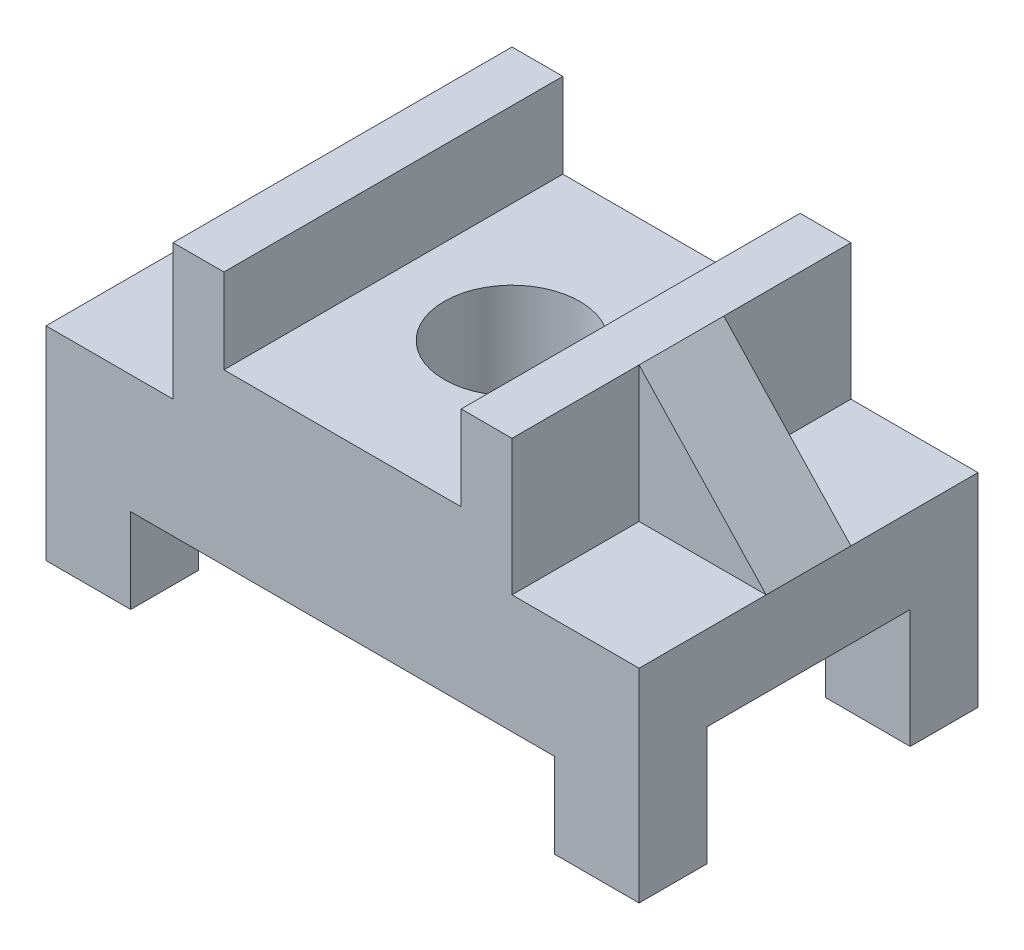
ISO-10303-21;
HEADER;
FILE_DESCRIPTION(('STEP AP214'),'2;1');
FILE_NAME('part.step','',(''),(''),'','','');
FILE_SCHEMA(('AUTOMOTIVE_DESIGN { 1 0 10303 214 1 1 1 1 }'));
ENDSEC;
DATA;
#1=APPLICATION_CONTEXT('core data for automotive mechanical design processes');
#2=APPLICATION_PROTOCOL_DEFINITION('international standard','automotive_design',2000,#1);
#3=PRODUCT_CONTEXT('',#1,'mechanical');
#4=PRODUCT('Part','Part','',(#3));
#5=PRODUCT_RELATED_PRODUCT_CATEGORY('part','',(#4));
#6=PRODUCT_DEFINITION_FORMATION('','',#4);
#7=PRODUCT_DEFINITION_CONTEXT('part definition',#1,'design');
#8=PRODUCT_DEFINITION('design','',#6,#7);
#9=PRODUCT_DEFINITION_SHAPE('','',#8);
#10=(LENGTH_UNIT() NAMED_UNIT(*) SI_UNIT(.MILLI.,.METRE.));
#11=(NAMED_UNIT(*) PLANE_ANGLE_UNIT() SI_UNIT($,.RADIAN.));
#12=(NAMED_UNIT(*) SI_UNIT($,.STERADIAN.) SOLID_ANGLE_UNIT());
#13=UNCERTAINTY_MEASURE_WITH_UNIT(LENGTH_MEASURE(1.E-05),#10,'distance_accuracy_value','');
#14=(GEOMETRIC_REPRESENTATION_CONTEXT(3) GLOBAL_UNCERTAINTY_ASSIGNED_CONTEXT((#13)) GLOBAL_UNIT_ASSIGNED_CONTEXT((#10,
#11,#12)) REPRESENTATION_CONTEXT('',''));
#15=CARTESIAN_POINT('',(0.,0.,0.));
#16=DIRECTION('',(0.,0.,1.));
#17=DIRECTION('',(1.,0.,0.));
#18=AXIS2_PLACEMENT_3D('',#15,#16,#17);
#19=CARTESIAN_POINT('',(0.,40.,20.));
#20=DIRECTION('',(0.,0.,-1.));
#21=DIRECTION('',(-1.,0.,0.));
#22=AXIS2_PLACEMENT_3D('',#19,#20,#21);
#23=PLANE('',#22);
#24=DIRECTION('',(0.,-1.,0.));
#25=VECTOR('',#24,1.);
#26=CARTESIAN_POINT('',(-25.,40.,20.));
#27=LINE('',#26,#25);
#28=CARTESIAN_POINT('',(-25.,10.,20.));
#29=VERTEX_POINT('',#28);
#30=CARTESIAN_POINT('',(-25.,0.,20.));
#31=VERTEX_POINT('',#30);
#32=EDGE_CURVE('E256',#29,#31,#27,.T.);
#33=ORIENTED_EDGE('',*,*,#32,.F.);
#34=DIRECTION('',(-1.,0.,0.));
#35=VECTOR('',#34,1.);
#36=CARTESIAN_POINT('',(0.,9.99999999999999,20.));
#37=LINE('',#36,#35);
#38=CARTESIAN_POINT('',(25.,10.,20.));
#39=VERTEX_POINT('',#38);
#40=EDGE_CURVE('E242',#39,#29,#37,.T.);
#41=ORIENTED_EDGE('',*,*,#40,.F.);
#42=DIRECTION('',(0.,1.,0.));
#43=VECTOR('',#42,1.);
#44=CARTESIAN_POINT('',(25.,40.,20.));
#45=LINE('',#44,#43);
#46=CARTESIAN_POINT('',(25.,0.,20.));
#47=VERTEX_POINT('',#46);
#48=EDGE_CURVE('E240',#47,#39,#45,.T.);
#49=ORIENTED_EDGE('',*,*,#48,.F.);
#50=DIRECTION('',(1.,0.,0.));
#51=VECTOR('',#50,1.);
#52=CARTESIAN_POINT('',(0.,0.,20.));
#53=LINE('',#52,#51);
#54=CARTESIAN_POINT('',(35.,0.,20.));
#55=VERTEX_POINT('',#54);
#56=EDGE_CURVE('E418',#47,#55,#53,.T.);
#57=ORIENTED_EDGE('',*,*,#56,.T.);
#58=DIRECTION('',(0.,-1.,0.));
#59=VECTOR('',#58,1.);
#60=CARTESIAN_POINT('',(35.,40.,20.));
#61=LINE('',#60,#59);
#62=CARTESIAN_POINT('',(35.,24.,20.));
#63=VERTEX_POINT('',#62);
#64=EDGE_CURVE('E432',#63,#55,#61,.T.);
#65=ORIENTED_EDGE('',*,*,#64,.F.);
#66=DIRECTION('',(1.,0.,0.));
#67=VECTOR('',#66,1.);
#68=CARTESIAN_POINT('',(0.,24.,20.));
#69=LINE('',#68,#67);
#70=CARTESIAN_POINT('',(20.,24.,20.));
#71=VERTEX_POINT('',#70);
#72=EDGE_CURVE('E360',#71,#63,#69,.T.);
#73=ORIENTED_EDGE('',*,*,#72,.F.);
#74=DIRECTION('',(0.,-1.,0.));
#75=VECTOR('',#74,1.);
#76=CARTESIAN_POINT('',(20.,40.,20.));
#77=LINE('',#76,#75);
#78=CARTESIAN_POINT('',(20.,40.,20.));
#79=VERTEX_POINT('',#78);
#80=EDGE_CURVE('E353',#79,#71,#77,.T.);
#81=ORIENTED_EDGE('',*,*,#80,.F.);
#82=DIRECTION('',(1.,0.,0.));
#83=VECTOR('',#82,1.);
#84=CARTESIAN_POINT('',(0.,40.,20.));
#85=LINE('',#84,#83);
#86=CARTESIAN_POINT('',(14.,40.,20.));
#87=VERTEX_POINT('',#86);
#88=EDGE_CURVE('E415',#87,#79,#85,.T.);
#89=ORIENTED_EDGE('',*,*,#88,.F.);
#90=DIRECTION('',(0.,1.,0.));
#91=VECTOR('',#90,1.);
#92=CARTESIAN_POINT('',(14.,0.,20.));
#93=LINE('',#92,#91);
#94=CARTESIAN_POINT('',(14.,30.,20.));
#95=VERTEX_POINT('',#94);
#96=EDGE_CURVE('E370',#95,#87,#93,.T.);
#97=ORIENTED_EDGE('',*,*,#96,.F.);
#98=DIRECTION('',(-1.,0.,0.));
#99=VECTOR('',#98,1.);
#100=CARTESIAN_POINT('',(0.,30.,20.));
#101=LINE('',#100,#99);
#102=CARTESIAN_POINT('',(-14.,30.,20.));
#103=VERTEX_POINT('',#102);
#104=EDGE_CURVE('E364',#95,#103,#101,.T.);
#105=ORIENTED_EDGE('',*,*,#104,.T.);
#106=DIRECTION('',(0.,1.,0.));
#107=VECTOR('',#106,1.);
#108=CARTESIAN_POINT('',(-14.,0.,20.));
#109=LINE('',#108,#107);
#110=CARTESIAN_POINT('',(-14.,40.,20.));
#111=VERTEX_POINT('',#110);
#112=EDGE_CURVE('E363',#103,#111,#109,.T.);
#113=ORIENTED_EDGE('',*,*,#112,.T.);
#114=CARTESIAN_POINT('',(-20.,40.,20.));
#115=VERTEX_POINT('',#114);
#116=EDGE_CURVE('E408',#115,#111,#85,.T.);
#117=ORIENTED_EDGE('',*,*,#116,.F.);
#118=DIRECTION('',(0.,1.,0.));
#119=VECTOR('',#118,1.);
#120=CARTESIAN_POINT('',(-20.,40.,20.));
#121=LINE('',#120,#119);
#122=CARTESIAN_POINT('',(-20.,24.,20.));
#123=VERTEX_POINT('',#122);
#124=EDGE_CURVE('E330',#123,#115,#121,.T.);
#125=ORIENTED_EDGE('',*,*,#124,.F.);
#126=DIRECTION('',(1.,0.,0.));
#127=VECTOR('',#126,1.);
#128=CARTESIAN_POINT('',(-35.,24.,20.));
#129=LINE('',#128,#127);
#130=CARTESIAN_POINT('',(-35.,24.,20.));
#131=VERTEX_POINT('',#130);
#132=EDGE_CURVE('E323',#131,#123,#129,.T.);
#133=ORIENTED_EDGE('',*,*,#132,.F.);
#134=DIRECTION('',(0.,-1.,0.));
#135=VECTOR('',#134,1.);
#136=CARTESIAN_POINT('',(-35.,40.,20.));
#137=LINE('',#136,#135);
#138=CARTESIAN_POINT('',(-35.,0.,20.));
#139=VERTEX_POINT('',#138);
#140=EDGE_CURVE('E440',#131,#139,#137,.T.);
#141=ORIENTED_EDGE('',*,*,#140,.T.);
#142=EDGE_CURVE('E420',#139,#31,#53,.T.);
#143=ORIENTED_EDGE('',*,*,#142,.T.);
#144=EDGE_LOOP('',(#33,#41,#49,#57,#65,#73,#81,#89,#97,#105,#113,#117,#125,#133,#141,#143));
#145=FACE_BOUND('',#144,.T.);
#146=ADVANCED_FACE('F43',(#145),#23,.F.);
#147=CARTESIAN_POINT('',(0.,0.,0.));
#148=DIRECTION('',(0.,1.,0.));
#149=DIRECTION('',(0.,0.,1.));
#150=AXIS2_PLACEMENT_3D('',#147,#148,#149);
#151=PLANE('',#150);
#152=DIRECTION('',(0.,0.,1.));
#153=VECTOR('',#152,1.);
#154=CARTESIAN_POINT('',(-25.,0.,-11.));
#155=LINE('',#154,#153);
#156=CARTESIAN_POINT('',(-25.,0.,12.));
#157=VERTEX_POINT('',#156);
#158=EDGE_CURVE('E244',#157,#31,#155,.T.);
#159=ORIENTED_EDGE('',*,*,#158,.T.);
#160=ORIENTED_EDGE('',*,*,#142,.F.);
#161=DIRECTION('',(0.,0.,1.));
#162=VECTOR('',#161,1.);
#163=CARTESIAN_POINT('',(-35.,0.,0.));
#164=LINE('',#163,#162);
#165=CARTESIAN_POINT('',(-35.,0.,12.));
#166=VERTEX_POINT('',#165);
#167=EDGE_CURVE('E400',#166,#139,#164,.T.);
#168=ORIENTED_EDGE('',*,*,#167,.F.);
#169=DIRECTION('',(-1.,0.,0.));
#170=VECTOR('',#169,1.);
#171=CARTESIAN_POINT('',(0.,0.,12.));
#172=LINE('',#171,#170);
#173=EDGE_CURVE('E396',#157,#166,#172,.T.);
#174=ORIENTED_EDGE('',*,*,#173,.F.);
#175=EDGE_LOOP('',(#159,#160,#168,#174));
#176=FACE_BOUND('',#175,.T.);
#177=ADVANCED_FACE('F518',(#176),#151,.F.);
#178=DIRECTION('',(0.,0.,1.));
#179=VECTOR('',#178,1.);
#180=CARTESIAN_POINT('',(25.,0.,-11.));
#181=LINE('',#180,#179);
#182=CARTESIAN_POINT('',(25.,0.,12.));
#183=VERTEX_POINT('',#182);
#184=EDGE_CURVE('E239',#183,#47,#181,.T.);
#185=ORIENTED_EDGE('',*,*,#184,.F.);
#186=CARTESIAN_POINT('',(35.,0.,12.));
#187=VERTEX_POINT('',#186);
#188=EDGE_CURVE('E409',#187,#183,#172,.T.);
#189=ORIENTED_EDGE('',*,*,#188,.F.);
#190=DIRECTION('',(0.,0.,-1.));
#191=VECTOR('',#190,1.);
#192=CARTESIAN_POINT('',(35.,0.,0.));
#193=LINE('',#192,#191);
#194=EDGE_CURVE('E421',#55,#187,#193,.T.);
#195=ORIENTED_EDGE('',*,*,#194,.F.);
#196=ORIENTED_EDGE('',*,*,#56,.F.);
#197=EDGE_LOOP('',(#185,#189,#195,#196));
#198=FACE_BOUND('',#197,.T.);
#199=ADVANCED_FACE('F469',(#198),#151,.F.);
#200=CARTESIAN_POINT('',(0.,14.,12.));
#201=DIRECTION('',(0.,0.,1.));
#202=DIRECTION('',(1.,0.,0.));
#203=AXIS2_PLACEMENT_3D('',#200,#201,#202);
#204=PLANE('',#203);
#205=DIRECTION('',(0.,1.,0.));
#206=VECTOR('',#205,1.);
#207=CARTESIAN_POINT('',(-25.,14.,12.));
#208=LINE('',#207,#206);
#209=CARTESIAN_POINT('',(-25.,10.,12.));
#210=VERTEX_POINT('',#209);
#211=EDGE_CURVE('E11',#157,#210,#208,.T.);
#212=ORIENTED_EDGE('',*,*,#211,.F.);
#213=ORIENTED_EDGE('',*,*,#173,.T.);
#214=DIRECTION('',(0.,1.,0.));
#215=VECTOR('',#214,1.);
#216=CARTESIAN_POINT('',(-35.,14.,12.));
#217=LINE('',#216,#215);
#218=CARTESIAN_POINT('',(-35.,14.,12.));
#219=VERTEX_POINT('',#218);
#220=EDGE_CURVE('E386',#166,#219,#217,.T.);
#221=ORIENTED_EDGE('',*,*,#220,.T.);
#222=DIRECTION('',(-1.,0.,0.));
#223=VECTOR('',#222,1.);
#224=CARTESIAN_POINT('',(0.,14.,12.));
#225=LINE('',#224,#223);
#226=CARTESIAN_POINT('',(35.,14.,12.));
#227=VERTEX_POINT('',#226);
#228=EDGE_CURVE('E404',#227,#219,#225,.T.);
#229=ORIENTED_EDGE('',*,*,#228,.F.);
#230=DIRECTION('',(0.,1.,0.));
#231=VECTOR('',#230,1.);
#232=CARTESIAN_POINT('',(35.,0.,12.));
#233=LINE('',#232,#231);
#234=EDGE_CURVE('E377',#187,#227,#233,.T.);
#235=ORIENTED_EDGE('',*,*,#234,.F.);
#236=ORIENTED_EDGE('',*,*,#188,.T.);
#237=DIRECTION('',(0.,-1.,0.));
#238=VECTOR('',#237,1.);
#239=CARTESIAN_POINT('',(25.,14.,12.));
#240=LINE('',#239,#238);
#241=CARTESIAN_POINT('',(25.,10.,12.));
#242=VERTEX_POINT('',#241);
#243=EDGE_CURVE('E467',#242,#183,#240,.T.);
#244=ORIENTED_EDGE('',*,*,#243,.F.);
#245=DIRECTION('',(1.,0.,0.));
#246=VECTOR('',#245,1.);
#247=CARTESIAN_POINT('',(0.,10.,12.));
#248=LINE('',#247,#246);
#249=EDGE_CURVE('E51',#210,#242,#248,.T.);
#250=ORIENTED_EDGE('',*,*,#249,.F.);
#251=EDGE_LOOP('',(#212,#213,#221,#229,#235,#236,#244,#250));
#252=FACE_BOUND('',#251,.T.);
#253=ADVANCED_FACE('F473',(#252),#204,.F.);
#254=DIRECTION('',(-1.,0.,0.));
#255=VECTOR('',#254,1.);
#256=CARTESIAN_POINT('',(0.,0.,-20.));
#257=LINE('',#256,#255);
#258=CARTESIAN_POINT('',(-25.,0.,-20.));
#259=VERTEX_POINT('',#258);
#260=CARTESIAN_POINT('',(-35.,0.,-20.));
#261=VERTEX_POINT('',#260);
#262=EDGE_CURVE('E428',#259,#261,#257,.T.);
#263=ORIENTED_EDGE('',*,*,#262,.F.);
#264=DIRECTION('',(0.,0.,1.));
#265=VECTOR('',#264,1.);
#266=CARTESIAN_POINT('',(-25.,0.,-43.));
#267=LINE('',#266,#265);
#268=CARTESIAN_POINT('',(-25.,0.,-12.));
#269=VERTEX_POINT('',#268);
#270=EDGE_CURVE('E268',#259,#269,#267,.T.);
#271=ORIENTED_EDGE('',*,*,#270,.T.);
#272=DIRECTION('',(-1.,0.,0.));
#273=VECTOR('',#272,1.);
#274=CARTESIAN_POINT('',(0.,0.,-12.));
#275=LINE('',#274,#273);
#276=CARTESIAN_POINT('',(-35.,0.,-12.));
#277=VERTEX_POINT('',#276);
#278=EDGE_CURVE('E402',#269,#277,#275,.T.);
#279=ORIENTED_EDGE('',*,*,#278,.T.);
#280=EDGE_CURVE('E416',#261,#277,#164,.T.);
#281=ORIENTED_EDGE('',*,*,#280,.F.);
#282=EDGE_LOOP('',(#263,#271,#279,#281));
#283=FACE_BOUND('',#282,.T.);
#284=ADVANCED_FACE('F540',(#283),#151,.F.);
#285=CARTESIAN_POINT('',(0.,24.,20.000012));
#286=DIRECTION('',(0.,1.,0.));
#287=DIRECTION('',(0.,0.,1.));
#288=AXIS2_PLACEMENT_3D('',#285,#286,#287);
#289=PLANE('',#288);
#290=DIRECTION('',(0.,0.,-1.));
#291=VECTOR('',#290,1.);
#292=CARTESIAN_POINT('',(35.,24.,20.000012));
#293=LINE('',#292,#291);
#294=CARTESIAN_POINT('',(35.,24.,5.00000000000001));
#295=VERTEX_POINT('',#294);
#296=EDGE_CURVE('E342',#63,#295,#293,.T.);
#297=ORIENTED_EDGE('',*,*,#296,.T.);
#298=DIRECTION('',(1.,0.,0.));
#299=VECTOR('',#298,1.);
#300=CARTESIAN_POINT('',(0.,24.,5.00000000000001));
#301=LINE('',#300,#299);
#302=CARTESIAN_POINT('',(20.,24.,5.00000000000001));
#303=VERTEX_POINT('',#302);
#304=EDGE_CURVE('E293',#303,#295,#301,.T.);
#305=ORIENTED_EDGE('',*,*,#304,.F.);
#306=DIRECTION('',(0.,0.,-1.));
#307=VECTOR('',#306,1.);
#308=CARTESIAN_POINT('',(20.,24.,20.000012));
#309=LINE('',#308,#307);
#310=EDGE_CURVE('E348',#71,#303,#309,.T.);
#311=ORIENTED_EDGE('',*,*,#310,.F.);
#312=ORIENTED_EDGE('',*,*,#72,.T.);
#313=EDGE_LOOP('',(#297,#305,#311,#312));
#314=FACE_BOUND('',#313,.T.);
#315=ADVANCED_FACE('F486',(#314),#289,.T.);
#316=CARTESIAN_POINT('',(20.,0.,20.000012));
#317=DIRECTION('',(1.,0.,0.));
#318=DIRECTION('',(0.,1.,0.));
#319=AXIS2_PLACEMENT_3D('',#316,#317,#318);
#320=PLANE('',#319);
#321=ORIENTED_EDGE('',*,*,#310,.T.);
#322=DIRECTION('',(0.,-1.,0.));
#323=VECTOR('',#322,1.);
#324=CARTESIAN_POINT('',(20.,40.,5.00000000000001));
#325=LINE('',#324,#323);
#326=CARTESIAN_POINT('',(20.,40.,5.00000000000001));
#327=VERTEX_POINT('',#326);
#328=EDGE_CURVE('E297',#327,#303,#325,.T.);
#329=ORIENTED_EDGE('',*,*,#328,.F.);
#330=DIRECTION('',(0.,0.,-1.));
#331=VECTOR('',#330,1.);
#332=CARTESIAN_POINT('',(20.,40.,0.));
#333=LINE('',#332,#331);
#334=EDGE_CURVE('E449',#79,#327,#333,.T.);
#335=ORIENTED_EDGE('',*,*,#334,.F.);
#336=ORIENTED_EDGE('',*,*,#80,.T.);
#337=EDGE_LOOP('',(#321,#329,#335,#336));
#338=FACE_BOUND('',#337,.T.);
#339=ADVANCED_FACE('F491',(#338),#320,.T.);
#340=CARTESIAN_POINT('',(-20.,40.,-75.));
#341=DIRECTION('',(1.,0.,0.));
#342=DIRECTION('',(0.,0.,-1.));
#343=AXIS2_PLACEMENT_3D('',#340,#341,#342);
#344=PLANE('',#343);
#345=DIRECTION('',(0.,-1.,0.));
#346=VECTOR('',#345,1.);
#347=CARTESIAN_POINT('',(-20.,40.,5.));
#348=LINE('',#347,#346);
#349=CARTESIAN_POINT('',(-20.,40.,5.));
#350=VERTEX_POINT('',#349);
#351=CARTESIAN_POINT('',(-20.,24.,5.));
#352=VERTEX_POINT('',#351);
#353=EDGE_CURVE('E324',#350,#352,#348,.T.);
#354=ORIENTED_EDGE('',*,*,#353,.T.);
#355=DIRECTION('',(0.,0.,1.));
#356=VECTOR('',#355,1.);
#357=CARTESIAN_POINT('',(-20.,24.,-75.));
#358=LINE('',#357,#356);
#359=EDGE_CURVE('E329',#352,#123,#358,.T.);
#360=ORIENTED_EDGE('',*,*,#359,.T.);
#361=ORIENTED_EDGE('',*,*,#124,.T.);
#362=DIRECTION('',(0.,0.,1.));
#363=VECTOR('',#362,1.);
#364=CARTESIAN_POINT('',(-20.,40.,-75.));
#365=LINE('',#364,#363);
#366=EDGE_CURVE('E335',#350,#115,#365,.T.);
#367=ORIENTED_EDGE('',*,*,#366,.F.);
#368=EDGE_LOOP('',(#354,#360,#361,#367));
#369=FACE_BOUND('',#368,.T.);
#370=ADVANCED_FACE('F576',(#369),#344,.F.);
#371=CARTESIAN_POINT('',(-35.,24.,-75.));
#372=DIRECTION('',(0.,-1.,0.));
#373=DIRECTION('',(0.,0.,-1.));
#374=AXIS2_PLACEMENT_3D('',#371,#372,#373);
#375=PLANE('',#374);
#376=DIRECTION('',(1.,0.,0.));
#377=VECTOR('',#376,1.);
#378=CARTESIAN_POINT('',(0.,24.,5.));
#379=LINE('',#378,#377);
#380=CARTESIAN_POINT('',(-35.,24.,5.));
#381=VERTEX_POINT('',#380);
#382=EDGE_CURVE('E313',#381,#352,#379,.T.);
#383=ORIENTED_EDGE('',*,*,#382,.F.);
#384=DIRECTION('',(0.,0.,-1.));
#385=VECTOR('',#384,1.);
#386=CARTESIAN_POINT('',(-35.,24.,0.));
#387=LINE('',#386,#385);
#388=EDGE_CURVE('E454',#131,#381,#387,.T.);
#389=ORIENTED_EDGE('',*,*,#388,.F.);
#390=ORIENTED_EDGE('',*,*,#132,.T.);
#391=ORIENTED_EDGE('',*,*,#359,.F.);
#392=EDGE_LOOP('',(#383,#389,#390,#391));
#393=FACE_BOUND('',#392,.T.);
#394=ADVANCED_FACE('F535',(#393),#375,.F.);
#395=CARTESIAN_POINT('',(0.,40.,-20.));
#396=DIRECTION('',(0.,0.,1.));
#397=DIRECTION('',(1.,0.,0.));
#398=AXIS2_PLACEMENT_3D('',#395,#396,#397);
#399=PLANE('',#398);
#400=DIRECTION('',(-1.,0.,0.));
#401=VECTOR('',#400,1.);
#402=CARTESIAN_POINT('',(0.,9.99999999999999,-20.));
#403=LINE('',#402,#401);
#404=CARTESIAN_POINT('',(25.,10.,-20.));
#405=VERTEX_POINT('',#404);
#406=CARTESIAN_POINT('',(-25.,10.,-20.));
#407=VERTEX_POINT('',#406);
#408=EDGE_CURVE('E273',#405,#407,#403,.T.);
#409=ORIENTED_EDGE('',*,*,#408,.T.);
#410=DIRECTION('',(0.,-1.,0.));
#411=VECTOR('',#410,1.);
#412=CARTESIAN_POINT('',(-25.,40.,-20.));
#413=LINE('',#412,#411);
#414=EDGE_CURVE('E280',#407,#259,#413,.T.);
#415=ORIENTED_EDGE('',*,*,#414,.T.);
#416=ORIENTED_EDGE('',*,*,#262,.T.);
#417=DIRECTION('',(0.,-1.,0.));
#418=VECTOR('',#417,1.);
#419=CARTESIAN_POINT('',(-35.,40.,-20.));
#420=LINE('',#419,#418);
#421=CARTESIAN_POINT('',(-35.,24.,-20.));
#422=VERTEX_POINT('',#421);
#423=EDGE_CURVE('E414',#422,#261,#420,.T.);
#424=ORIENTED_EDGE('',*,*,#423,.F.);
#425=DIRECTION('',(1.,0.,0.));
#426=VECTOR('',#425,1.);
#427=CARTESIAN_POINT('',(0.,24.,-20.));
#428=LINE('',#427,#426);
#429=CARTESIAN_POINT('',(-20.,24.,-20.));
#430=VERTEX_POINT('',#429);
#431=EDGE_CURVE('E333',#422,#430,#428,.T.);
#432=ORIENTED_EDGE('',*,*,#431,.T.);
#433=DIRECTION('',(0.,1.,0.));
#434=VECTOR('',#433,1.);
#435=CARTESIAN_POINT('',(-20.,40.,-20.));
#436=LINE('',#435,#434);
#437=CARTESIAN_POINT('',(-20.,40.,-20.));
#438=VERTEX_POINT('',#437);
#439=EDGE_CURVE('E344',#430,#438,#436,.T.);
#440=ORIENTED_EDGE('',*,*,#439,.T.);
#441=DIRECTION('',(-1.,0.,0.));
#442=VECTOR('',#441,1.);
#443=CARTESIAN_POINT('',(0.,40.,-20.));
#444=LINE('',#443,#442);
#445=CARTESIAN_POINT('',(-14.,40.,-20.));
#446=VERTEX_POINT('',#445);
#447=EDGE_CURVE('E411',#446,#438,#444,.T.);
#448=ORIENTED_EDGE('',*,*,#447,.F.);
#449=DIRECTION('',(0.,1.,0.));
#450=VECTOR('',#449,1.);
#451=CARTESIAN_POINT('',(-14.,40.,-20.));
#452=LINE('',#451,#450);
#453=CARTESIAN_POINT('',(-14.,30.,-20.));
#454=VERTEX_POINT('',#453);
#455=EDGE_CURVE('E376',#454,#446,#452,.T.);
#456=ORIENTED_EDGE('',*,*,#455,.F.);
#457=DIRECTION('',(-1.,0.,0.));
#458=VECTOR('',#457,1.);
#459=CARTESIAN_POINT('',(0.,30.,-20.));
#460=LINE('',#459,#458);
#461=CARTESIAN_POINT('',(14.,30.,-20.));
#462=VERTEX_POINT('',#461);
#463=EDGE_CURVE('E444',#462,#454,#460,.T.);
#464=ORIENTED_EDGE('',*,*,#463,.F.);
#465=DIRECTION('',(0.,1.,0.));
#466=VECTOR('',#465,1.);
#467=CARTESIAN_POINT('',(14.,40.,-20.));
#468=LINE('',#467,#466);
#469=CARTESIAN_POINT('',(14.,40.,-20.));
#470=VERTEX_POINT('',#469);
#471=EDGE_CURVE('E375',#462,#470,#468,.T.);
#472=ORIENTED_EDGE('',*,*,#471,.T.);
#473=CARTESIAN_POINT('',(20.,40.,-20.));
#474=VERTEX_POINT('',#473);
#475=EDGE_CURVE('E413',#474,#470,#444,.T.);
#476=ORIENTED_EDGE('',*,*,#475,.F.);
#477=DIRECTION('',(0.,1.,0.));
#478=VECTOR('',#477,1.);
#479=CARTESIAN_POINT('',(20.,40.,-20.));
#480=LINE('',#479,#478);
#481=CARTESIAN_POINT('',(20.,24.,-20.));
#482=VERTEX_POINT('',#481);
#483=EDGE_CURVE('E351',#482,#474,#480,.T.);
#484=ORIENTED_EDGE('',*,*,#483,.F.);
#485=DIRECTION('',(-1.,0.,0.));
#486=VECTOR('',#485,1.);
#487=CARTESIAN_POINT('',(0.,24.,-20.));
#488=LINE('',#487,#486);
#489=CARTESIAN_POINT('',(35.,24.,-20.));
#490=VERTEX_POINT('',#489);
#491=EDGE_CURVE('E358',#490,#482,#488,.T.);
#492=ORIENTED_EDGE('',*,*,#491,.F.);
#493=DIRECTION('',(0.,-1.,0.));
#494=VECTOR('',#493,1.);
#495=CARTESIAN_POINT('',(35.,40.,-20.));
#496=LINE('',#495,#494);
#497=CARTESIAN_POINT('',(35.,0.,-20.));
#498=VERTEX_POINT('',#497);
#499=EDGE_CURVE('E435',#490,#498,#496,.T.);
#500=ORIENTED_EDGE('',*,*,#499,.T.);
#501=CARTESIAN_POINT('',(25.,0.,-20.));
#502=VERTEX_POINT('',#501);
#503=EDGE_CURVE('E430',#498,#502,#257,.T.);
#504=ORIENTED_EDGE('',*,*,#503,.T.);
#505=DIRECTION('',(0.,1.,0.));
#506=VECTOR('',#505,1.);
#507=CARTESIAN_POINT('',(25.,40.,-20.));
#508=LINE('',#507,#506);
#509=EDGE_CURVE('E275',#502,#405,#508,.T.);
#510=ORIENTED_EDGE('',*,*,#509,.T.);
#511=EDGE_LOOP('',(#409,#415,#416,#424,#432,#440,#448,#456,#464,#472,#476,#484,#492,#500,#504,#510));
#512=FACE_BOUND('',#511,.T.);
#513=ADVANCED_FACE('F530',(#512),#399,.F.);
#514=CARTESIAN_POINT('',(35.,40.,0.));
#515=DIRECTION('',(-1.,0.,0.));
#516=DIRECTION('',(0.,0.,1.));
#517=AXIS2_PLACEMENT_3D('',#514,#515,#516);
#518=PLANE('',#517);
#519=CARTESIAN_POINT('',(35.,24.,-4.99999999999999));
#520=VERTEX_POINT('',#519);
#521=EDGE_CURVE('E343',#520,#490,#293,.T.);
#522=ORIENTED_EDGE('',*,*,#521,.F.);
#523=DIRECTION('',(0.,0.,-1.));
#524=VECTOR('',#523,1.);
#525=CARTESIAN_POINT('',(35.,24.,11.));
#526=LINE('',#525,#524);
#527=EDGE_CURVE('E283',#295,#520,#526,.T.);
#528=ORIENTED_EDGE('',*,*,#527,.F.);
#529=ORIENTED_EDGE('',*,*,#296,.F.);
#530=ORIENTED_EDGE('',*,*,#64,.T.);
#531=ORIENTED_EDGE('',*,*,#194,.T.);
#532=ORIENTED_EDGE('',*,*,#234,.T.);
#533=DIRECTION('',(0.,0.,-1.));
#534=VECTOR('',#533,1.);
#535=CARTESIAN_POINT('',(35.,14.,12.));
#536=LINE('',#535,#534);
#537=CARTESIAN_POINT('',(35.,14.,-12.));
#538=VERTEX_POINT('',#537);
#539=EDGE_CURVE('E382',#227,#538,#536,.T.);
#540=ORIENTED_EDGE('',*,*,#539,.T.);
#541=DIRECTION('',(0.,-1.,0.));
#542=VECTOR('',#541,1.);
#543=CARTESIAN_POINT('',(35.,0.,-12.));
#544=LINE('',#543,#542);
#545=CARTESIAN_POINT('',(35.,0.,-12.));
#546=VERTEX_POINT('',#545);
#547=EDGE_CURVE('E381',#538,#546,#544,.T.);
#548=ORIENTED_EDGE('',*,*,#547,.T.);
#549=EDGE_CURVE('E422',#546,#498,#193,.T.);
#550=ORIENTED_EDGE('',*,*,#549,.T.);
#551=ORIENTED_EDGE('',*,*,#499,.F.);
#552=EDGE_LOOP('',(#522,#528,#529,#530,#531,#532,#540,#548,#550,#551));
#553=FACE_BOUND('',#552,.T.);
#554=ADVANCED_FACE('F478',(#553),#518,.F.);
#555=CARTESIAN_POINT('',(0.,40.,0.));
#556=DIRECTION('',(0.,1.,0.));
#557=DIRECTION('',(0.,0.,1.));
#558=AXIS2_PLACEMENT_3D('',#555,#556,#557);
#559=PLANE('',#558);
#560=DIRECTION('',(0.,0.,-1.));
#561=VECTOR('',#560,1.);
#562=CARTESIAN_POINT('',(20.,40.,11.));
#563=LINE('',#562,#561);
#564=CARTESIAN_POINT('',(20.,40.,-4.99999999999999));
#565=VERTEX_POINT('',#564);
#566=EDGE_CURVE('E282',#327,#565,#563,.T.);
#567=ORIENTED_EDGE('',*,*,#566,.T.);
#568=EDGE_CURVE('E450',#565,#474,#333,.T.);
#569=ORIENTED_EDGE('',*,*,#568,.T.);
#570=ORIENTED_EDGE('',*,*,#475,.T.);
#571=DIRECTION('',(0.,0.,-1.));
#572=VECTOR('',#571,1.);
#573=CARTESIAN_POINT('',(14.,40.,0.));
#574=LINE('',#573,#572);
#575=EDGE_CURVE('E437',#87,#470,#574,.T.);
#576=ORIENTED_EDGE('',*,*,#575,.F.);
#577=ORIENTED_EDGE('',*,*,#88,.T.);
#578=ORIENTED_EDGE('',*,*,#334,.T.);
#579=EDGE_LOOP('',(#567,#569,#570,#576,#577,#578));
#580=FACE_BOUND('',#579,.T.);
#581=ADVANCED_FACE('F496',(#580),#559,.T.);
#582=DIRECTION('',(0.,0.,-1.));
#583=VECTOR('',#582,1.);
#584=CARTESIAN_POINT('',(-20.,40.,45.));
#585=LINE('',#584,#583);
#586=CARTESIAN_POINT('',(-20.,40.,-5.));
#587=VERTEX_POINT('',#586);
#588=EDGE_CURVE('E307',#350,#587,#585,.T.);
#589=ORIENTED_EDGE('',*,*,#588,.F.);
#590=ORIENTED_EDGE('',*,*,#366,.T.);
#591=ORIENTED_EDGE('',*,*,#116,.T.);
#592=DIRECTION('',(0.,0.,-1.));
#593=VECTOR('',#592,1.);
#594=CARTESIAN_POINT('',(-14.,40.,0.));
#595=LINE('',#594,#593);
#596=EDGE_CURVE('E445',#111,#446,#595,.T.);
#597=ORIENTED_EDGE('',*,*,#596,.T.);
#598=ORIENTED_EDGE('',*,*,#447,.T.);
#599=EDGE_CURVE('E331',#438,#587,#365,.T.);
#600=ORIENTED_EDGE('',*,*,#599,.T.);
#601=EDGE_LOOP('',(#589,#590,#591,#597,#598,#600));
#602=FACE_BOUND('',#601,.T.);
#603=ADVANCED_FACE('F541',(#602),#559,.T.);
#604=CARTESIAN_POINT('',(-35.,40.,0.));
#605=DIRECTION('',(1.,0.,0.));
#606=DIRECTION('',(0.,0.,-1.));
#607=AXIS2_PLACEMENT_3D('',#604,#605,#606);
#608=PLANE('',#607);
#609=ORIENTED_EDGE('',*,*,#388,.T.);
#610=DIRECTION('',(0.,0.,-1.));
#611=VECTOR('',#610,1.);
#612=CARTESIAN_POINT('',(-35.,24.,45.));
#613=LINE('',#612,#611);
#614=CARTESIAN_POINT('',(-35.,24.,-5.));
#615=VERTEX_POINT('',#614);
#616=EDGE_CURVE('E306',#381,#615,#613,.T.);
#617=ORIENTED_EDGE('',*,*,#616,.T.);
#618=EDGE_CURVE('E448',#615,#422,#387,.T.);
#619=ORIENTED_EDGE('',*,*,#618,.T.);
#620=ORIENTED_EDGE('',*,*,#423,.T.);
#621=ORIENTED_EDGE('',*,*,#280,.T.);
#622=DIRECTION('',(0.,-1.,0.));
#623=VECTOR('',#622,1.);
#624=CARTESIAN_POINT('',(-35.,0.,-12.));
#625=LINE('',#624,#623);
#626=CARTESIAN_POINT('',(-35.,14.,-12.));
#627=VERTEX_POINT('',#626);
#628=EDGE_CURVE('E393',#627,#277,#625,.T.);
#629=ORIENTED_EDGE('',*,*,#628,.F.);
#630=DIRECTION('',(0.,0.,-1.));
#631=VECTOR('',#630,1.);
#632=CARTESIAN_POINT('',(-35.,14.,-12.));
#633=LINE('',#632,#631);
#634=EDGE_CURVE('E387',#219,#627,#633,.T.);
#635=ORIENTED_EDGE('',*,*,#634,.F.);
#636=ORIENTED_EDGE('',*,*,#220,.F.);
#637=ORIENTED_EDGE('',*,*,#167,.T.);
#638=ORIENTED_EDGE('',*,*,#140,.F.);
#639=EDGE_LOOP('',(#609,#617,#619,#620,#621,#629,#635,#636,#637,#638));
#640=FACE_BOUND('',#639,.T.);
#641=ADVANCED_FACE('F44',(#640),#608,.F.);
#642=CARTESIAN_POINT('',(25.,0.,-12.));
#643=VERTEX_POINT('',#642);
#644=EDGE_CURVE('E397',#546,#643,#275,.T.);
#645=ORIENTED_EDGE('',*,*,#644,.T.);
#646=DIRECTION('',(0.,0.,1.));
#647=VECTOR('',#646,1.);
#648=CARTESIAN_POINT('',(25.,0.,-43.));
#649=LINE('',#648,#647);
#650=EDGE_CURVE('E66',#502,#643,#649,.T.);
#651=ORIENTED_EDGE('',*,*,#650,.F.);
#652=ORIENTED_EDGE('',*,*,#503,.F.);
#653=ORIENTED_EDGE('',*,*,#549,.F.);
#654=EDGE_LOOP('',(#645,#651,#652,#653));
#655=FACE_BOUND('',#654,.T.);
#656=ADVANCED_FACE('F526',(#655),#151,.F.);
#657=CARTESIAN_POINT('',(0.,0.,-12.));
#658=DIRECTION('',(0.,0.,-1.));
#659=DIRECTION('',(-1.,0.,0.));
#660=AXIS2_PLACEMENT_3D('',#657,#658,#659);
#661=PLANE('',#660);
#662=ORIENTED_EDGE('',*,*,#278,.F.);
#663=DIRECTION('',(0.,1.,0.));
#664=VECTOR('',#663,1.);
#665=CARTESIAN_POINT('',(-25.,0.,-12.));
#666=LINE('',#665,#664);
#667=CARTESIAN_POINT('',(-25.,10.,-12.));
#668=VERTEX_POINT('',#667);
#669=EDGE_CURVE('E464',#269,#668,#666,.T.);
#670=ORIENTED_EDGE('',*,*,#669,.T.);
#671=DIRECTION('',(1.,0.,0.));
#672=VECTOR('',#671,1.);
#673=CARTESIAN_POINT('',(0.,10.,-12.));
#674=LINE('',#673,#672);
#675=CARTESIAN_POINT('',(25.,10.,-12.));
#676=VERTEX_POINT('',#675);
#677=EDGE_CURVE('E459',#668,#676,#674,.T.);
#678=ORIENTED_EDGE('',*,*,#677,.T.);
#679=DIRECTION('',(0.,-1.,0.));
#680=VECTOR('',#679,1.);
#681=CARTESIAN_POINT('',(25.,0.,-12.));
#682=LINE('',#681,#680);
#683=EDGE_CURVE('E456',#676,#643,#682,.T.);
#684=ORIENTED_EDGE('',*,*,#683,.T.);
#685=ORIENTED_EDGE('',*,*,#644,.F.);
#686=ORIENTED_EDGE('',*,*,#547,.F.);
#687=DIRECTION('',(-1.,0.,0.));
#688=VECTOR('',#687,1.);
#689=CARTESIAN_POINT('',(0.,14.,-12.));
#690=LINE('',#689,#688);
#691=EDGE_CURVE('E405',#538,#627,#690,.T.);
#692=ORIENTED_EDGE('',*,*,#691,.T.);
#693=ORIENTED_EDGE('',*,*,#628,.T.);
#694=EDGE_LOOP('',(#662,#670,#678,#684,#685,#686,#692,#693));
#695=FACE_BOUND('',#694,.T.);
#696=ADVANCED_FACE('F539',(#695),#661,.F.);
#697=CARTESIAN_POINT('',(0.,14.,-12.));
#698=DIRECTION('',(0.,1.,0.));
#699=DIRECTION('',(0.,0.,1.));
#700=AXIS2_PLACEMENT_3D('',#697,#698,#699);
#701=PLANE('',#700);
#702=CARTESIAN_POINT('',(0.,14.,0.));
#703=DIRECTION('',(0.,1.,0.));
#704=DIRECTION('',(0.,0.,1.));
#705=AXIS2_PLACEMENT_3D('',#702,#703,#704);
#706=CIRCLE('',#705,8.);
#707=CARTESIAN_POINT('',(0.,14.,8.));
#708=VERTEX_POINT('',#707);
#709=EDGE_CURVE('E303',#708,#708,#706,.F.);
#710=ORIENTED_EDGE('',*,*,#709,.F.);
#711=EDGE_LOOP('',(#710));
#712=FACE_BOUND('',#711,.T.);
#713=ORIENTED_EDGE('',*,*,#634,.T.);
#714=ORIENTED_EDGE('',*,*,#691,.F.);
#715=ORIENTED_EDGE('',*,*,#539,.F.);
#716=ORIENTED_EDGE('',*,*,#228,.T.);
#717=EDGE_LOOP('',(#713,#714,#715,#716));
#718=FACE_BOUND('',#717,.T.);
#719=ADVANCED_FACE('F542',(#712,#718),#701,.F.);
#720=CARTESIAN_POINT('',(0.,30.,-29.));
#721=DIRECTION('',(0.,1.,0.));
#722=DIRECTION('',(-1.,0.,0.));
#723=AXIS2_PLACEMENT_3D('',#720,#721,#722);
#724=PLANE('',#723);
#725=CARTESIAN_POINT('',(0.,30.,0.));
#726=DIRECTION('',(0.,1.,0.));
#727=DIRECTION('',(-1.,0.,0.));
#728=AXIS2_PLACEMENT_3D('',#725,#726,#727);
#729=CIRCLE('',#728,8.);
#730=CARTESIAN_POINT('',(-8.00000000000001,30.,0.));
#731=VERTEX_POINT('',#730);
#732=EDGE_CURVE('E305',#731,#731,#729,.F.);
#733=ORIENTED_EDGE('',*,*,#732,.T.);
#734=EDGE_LOOP('',(#733));
#735=FACE_BOUND('',#734,.T.);
#736=ORIENTED_EDGE('',*,*,#463,.T.);
#737=DIRECTION('',(0.,0.,1.));
#738=VECTOR('',#737,1.);
#739=CARTESIAN_POINT('',(-14.,30.,-29.));
#740=LINE('',#739,#738);
#741=EDGE_CURVE('E367',#454,#103,#740,.T.);
#742=ORIENTED_EDGE('',*,*,#741,.T.);
#743=ORIENTED_EDGE('',*,*,#104,.F.);
#744=DIRECTION('',(0.,0.,1.));
#745=VECTOR('',#744,1.);
#746=CARTESIAN_POINT('',(14.,30.,-29.));
#747=LINE('',#746,#745);
#748=EDGE_CURVE('E369',#462,#95,#747,.T.);
#749=ORIENTED_EDGE('',*,*,#748,.F.);
#750=EDGE_LOOP('',(#736,#742,#743,#749));
#751=FACE_BOUND('',#750,.T.);
#752=ADVANCED_FACE('F547',(#735,#751),#724,.T.);
#753=CARTESIAN_POINT('',(-14.,0.,-29.));
#754=DIRECTION('',(1.,0.,0.));
#755=DIRECTION('',(0.,0.,-1.));
#756=AXIS2_PLACEMENT_3D('',#753,#754,#755);
#757=PLANE('',#756);
#758=ORIENTED_EDGE('',*,*,#455,.T.);
#759=ORIENTED_EDGE('',*,*,#596,.F.);
#760=ORIENTED_EDGE('',*,*,#112,.F.);
#761=ORIENTED_EDGE('',*,*,#741,.F.);
#762=EDGE_LOOP('',(#758,#759,#760,#761));
#763=FACE_BOUND('',#762,.T.);
#764=ADVANCED_FACE('F552',(#763),#757,.T.);
#765=CARTESIAN_POINT('',(14.,0.,-29.));
#766=DIRECTION('',(1.,0.,0.));
#767=DIRECTION('',(0.,0.,-1.));
#768=AXIS2_PLACEMENT_3D('',#765,#766,#767);
#769=PLANE('',#768);
#770=ORIENTED_EDGE('',*,*,#748,.T.);
#771=ORIENTED_EDGE('',*,*,#96,.T.);
#772=ORIENTED_EDGE('',*,*,#575,.T.);
#773=ORIENTED_EDGE('',*,*,#471,.F.);
#774=EDGE_LOOP('',(#770,#771,#772,#773));
#775=FACE_BOUND('',#774,.T.);
#776=ADVANCED_FACE('F554',(#775),#769,.F.);
#777=DIRECTION('',(1.,0.,0.));
#778=VECTOR('',#777,1.);
#779=CARTESIAN_POINT('',(0.,24.,-4.99999999999999));
#780=LINE('',#779,#778);
#781=CARTESIAN_POINT('',(20.,24.,-4.99999999999999));
#782=VERTEX_POINT('',#781);
#783=EDGE_CURVE('E295',#782,#520,#780,.T.);
#784=ORIENTED_EDGE('',*,*,#783,.T.);
#785=ORIENTED_EDGE('',*,*,#521,.T.);
#786=ORIENTED_EDGE('',*,*,#491,.T.);
#787=EDGE_CURVE('E350',#782,#482,#309,.T.);
#788=ORIENTED_EDGE('',*,*,#787,.F.);
#789=EDGE_LOOP('',(#784,#785,#786,#788));
#790=FACE_BOUND('',#789,.T.);
#791=ADVANCED_FACE('F565',(#790),#289,.T.);
#792=DIRECTION('',(0.,-1.,0.));
#793=VECTOR('',#792,1.);
#794=CARTESIAN_POINT('',(20.,40.,-4.99999999999999));
#795=LINE('',#794,#793);
#796=EDGE_CURVE('E300',#565,#782,#795,.T.);
#797=ORIENTED_EDGE('',*,*,#796,.T.);
#798=ORIENTED_EDGE('',*,*,#787,.T.);
#799=ORIENTED_EDGE('',*,*,#483,.T.);
#800=ORIENTED_EDGE('',*,*,#568,.F.);
#801=EDGE_LOOP('',(#797,#798,#799,#800));
#802=FACE_BOUND('',#801,.T.);
#803=ADVANCED_FACE('F562',(#802),#320,.T.);
#804=CARTESIAN_POINT('',(-20.,24.,-5.));
#805=VERTEX_POINT('',#804);
#806=EDGE_CURVE('E337',#430,#805,#358,.T.);
#807=ORIENTED_EDGE('',*,*,#806,.T.);
#808=DIRECTION('',(0.,-1.,0.));
#809=VECTOR('',#808,1.);
#810=CARTESIAN_POINT('',(-20.,40.,-5.));
#811=LINE('',#810,#809);
#812=EDGE_CURVE('E316',#587,#805,#811,.T.);
#813=ORIENTED_EDGE('',*,*,#812,.F.);
#814=ORIENTED_EDGE('',*,*,#599,.F.);
#815=ORIENTED_EDGE('',*,*,#439,.F.);
#816=EDGE_LOOP('',(#807,#813,#814,#815));
#817=FACE_BOUND('',#816,.T.);
#818=ADVANCED_FACE('F566',(#817),#344,.F.);
#819=ORIENTED_EDGE('',*,*,#618,.F.);
#820=DIRECTION('',(1.,0.,0.));
#821=VECTOR('',#820,1.);
#822=CARTESIAN_POINT('',(0.,24.,-5.));
#823=LINE('',#822,#821);
#824=EDGE_CURVE('E317',#615,#805,#823,.T.);
#825=ORIENTED_EDGE('',*,*,#824,.T.);
#826=ORIENTED_EDGE('',*,*,#806,.F.);
#827=ORIENTED_EDGE('',*,*,#431,.F.);
#828=EDGE_LOOP('',(#819,#825,#826,#827));
#829=FACE_BOUND('',#828,.T.);
#830=ADVANCED_FACE('F571',(#829),#375,.F.);
#831=CARTESIAN_POINT('',(0.,40.,5.));
#832=DIRECTION('',(0.,0.,-1.));
#833=DIRECTION('',(-1.,0.,0.));
#834=AXIS2_PLACEMENT_3D('',#831,#832,#833);
#835=PLANE('',#834);
#836=ORIENTED_EDGE('',*,*,#353,.F.);
#837=DIRECTION('',(-0.68394112888133,-0.729537204140085,0.));
#838=VECTOR('',#837,1.);
#839=CARTESIAN_POINT('',(-10.6444906444906,49.97920997921,5.));
#840=LINE('',#839,#838);
#841=EDGE_CURVE('E311',#350,#381,#840,.T.);
#842=ORIENTED_EDGE('',*,*,#841,.T.);
#843=ORIENTED_EDGE('',*,*,#382,.T.);
#844=EDGE_LOOP('',(#836,#842,#843));
#845=FACE_BOUND('',#844,.T.);
#846=ADVANCED_FACE('F573',(#845),#835,.F.);
#847=CARTESIAN_POINT('',(0.,40.,-5.));
#848=DIRECTION('',(0.,0.,-1.));
#849=DIRECTION('',(-1.,0.,0.));
#850=AXIS2_PLACEMENT_3D('',#847,#848,#849);
#851=PLANE('',#850);
#852=DIRECTION('',(-0.68394112888133,-0.729537204140085,0.));
#853=VECTOR('',#852,1.);
#854=CARTESIAN_POINT('',(-10.6444906444906,49.97920997921,-5.));
#855=LINE('',#854,#853);
#856=EDGE_CURVE('E453',#587,#615,#855,.T.);
#857=ORIENTED_EDGE('',*,*,#856,.F.);
#858=ORIENTED_EDGE('',*,*,#812,.T.);
#859=ORIENTED_EDGE('',*,*,#824,.F.);
#860=EDGE_LOOP('',(#857,#858,#859));
#861=FACE_BOUND('',#860,.T.);
#862=ADVANCED_FACE('F581',(#861),#851,.T.);
#863=CARTESIAN_POINT('',(-30.6029106029106,28.6902286902287,45.));
#864=DIRECTION('',(0.729537204140085,-0.68394112888133,0.));
#865=DIRECTION('',(0.68394112888133,0.729537204140085,0.));
#866=AXIS2_PLACEMENT_3D('',#863,#864,#865);
#867=PLANE('',#866);
#868=ORIENTED_EDGE('',*,*,#588,.T.);
#869=ORIENTED_EDGE('',*,*,#856,.T.);
#870=ORIENTED_EDGE('',*,*,#616,.F.);
#871=ORIENTED_EDGE('',*,*,#841,.F.);
#872=EDGE_LOOP('',(#868,#869,#870,#871));
#873=FACE_BOUND('',#872,.T.);
#874=ADVANCED_FACE('F513',(#873),#867,.F.);
#875=CARTESIAN_POINT('',(0.,82.,0.));
#876=DIRECTION('',(0.,-1.,0.));
#877=DIRECTION('',(1.,0.,0.));
#878=AXIS2_PLACEMENT_3D('',#875,#876,#877);
#879=CYLINDRICAL_SURFACE('',#878,8.);
#880=ORIENTED_EDGE('',*,*,#732,.F.);
#881=EDGE_LOOP('',(#880));
#882=FACE_BOUND('',#881,.T.);
#883=ORIENTED_EDGE('',*,*,#709,.T.);
#884=EDGE_LOOP('',(#883));
#885=FACE_BOUND('',#884,.T.);
#886=ADVANCED_FACE('F506',(#882,#885),#879,.F.);
#887=CARTESIAN_POINT('',(0.,40.,5.00000000000001));
#888=DIRECTION('',(0.,0.,-1.));
#889=DIRECTION('',(-1.,0.,0.));
#890=AXIS2_PLACEMENT_3D('',#887,#888,#889);
#891=PLANE('',#890);
#892=ORIENTED_EDGE('',*,*,#304,.T.);
#893=DIRECTION('',(-0.68394112888133,0.729537204140085,0.));
#894=VECTOR('',#893,1.);
#895=CARTESIAN_POINT('',(10.6444906444906,49.97920997921,5.00000000000001));
#896=LINE('',#895,#894);
#897=EDGE_CURVE('E287',#295,#327,#896,.T.);
#898=ORIENTED_EDGE('',*,*,#897,.T.);
#899=ORIENTED_EDGE('',*,*,#328,.T.);
#900=EDGE_LOOP('',(#892,#898,#899));
#901=FACE_BOUND('',#900,.T.);
#902=ADVANCED_FACE('F503',(#901),#891,.F.);
#903=CARTESIAN_POINT('',(0.,40.,-4.99999999999999));
#904=DIRECTION('',(0.,0.,-1.));
#905=DIRECTION('',(-1.,0.,0.));
#906=AXIS2_PLACEMENT_3D('',#903,#904,#905);
#907=PLANE('',#906);
#908=DIRECTION('',(-0.68394112888133,0.729537204140085,0.));
#909=VECTOR('',#908,1.);
#910=CARTESIAN_POINT('',(20.,40.,-4.99999999999999));
#911=LINE('',#910,#909);
#912=EDGE_CURVE('E281',#520,#565,#911,.T.);
#913=ORIENTED_EDGE('',*,*,#912,.F.);
#914=ORIENTED_EDGE('',*,*,#783,.F.);
#915=ORIENTED_EDGE('',*,*,#796,.F.);
#916=EDGE_LOOP('',(#913,#914,#915));
#917=FACE_BOUND('',#916,.T.);
#918=ADVANCED_FACE('F504',(#917),#907,.T.);
#919=CARTESIAN_POINT('',(20.,40.,11.));
#920=DIRECTION('',(-0.729537204140085,-0.68394112888133,0.));
#921=DIRECTION('',(0.68394112888133,-0.729537204140085,0.));
#922=AXIS2_PLACEMENT_3D('',#919,#920,#921);
#923=PLANE('',#922);
#924=ORIENTED_EDGE('',*,*,#527,.T.);
#925=ORIENTED_EDGE('',*,*,#912,.T.);
#926=ORIENTED_EDGE('',*,*,#566,.F.);
#927=ORIENTED_EDGE('',*,*,#897,.F.);
#928=EDGE_LOOP('',(#924,#925,#926,#927));
#929=FACE_BOUND('',#928,.T.);
#930=ADVANCED_FACE('F499',(#929),#923,.F.);
#931=CARTESIAN_POINT('',(-25.,10.,-43.));
#932=DIRECTION('',(-1.,0.,0.));
#933=DIRECTION('',(0.,-1.,0.));
#934=AXIS2_PLACEMENT_3D('',#931,#932,#933);
#935=PLANE('',#934);
#936=DIRECTION('',(0.,0.,1.));
#937=VECTOR('',#936,1.);
#938=CARTESIAN_POINT('',(-25.,10.,-43.));
#939=LINE('',#938,#937);
#940=EDGE_CURVE('E266',#407,#668,#939,.T.);
#941=ORIENTED_EDGE('',*,*,#940,.T.);
#942=ORIENTED_EDGE('',*,*,#669,.F.);
#943=ORIENTED_EDGE('',*,*,#270,.F.);
#944=ORIENTED_EDGE('',*,*,#414,.F.);
#945=EDGE_LOOP('',(#941,#942,#943,#944));
#946=FACE_BOUND('',#945,.T.);
#947=ADVANCED_FACE('F639',(#946),#935,.F.);
#948=CARTESIAN_POINT('',(25.,10.,-43.));
#949=DIRECTION('',(0.,1.,0.));
#950=DIRECTION('',(0.,0.,1.));
#951=AXIS2_PLACEMENT_3D('',#948,#949,#950);
#952=PLANE('',#951);
#953=DIRECTION('',(0.,0.,1.));
#954=VECTOR('',#953,1.);
#955=CARTESIAN_POINT('',(25.,10.,-43.));
#956=LINE('',#955,#954);
#957=EDGE_CURVE('E263',#405,#676,#956,.T.);
#958=ORIENTED_EDGE('',*,*,#957,.T.);
#959=ORIENTED_EDGE('',*,*,#677,.F.);
#960=ORIENTED_EDGE('',*,*,#940,.F.);
#961=ORIENTED_EDGE('',*,*,#408,.F.);
#962=EDGE_LOOP('',(#958,#959,#960,#961));
#963=FACE_BOUND('',#962,.T.);
#964=ADVANCED_FACE('F636',(#963),#952,.F.);
#965=CARTESIAN_POINT('',(25.,0.,-43.));
#966=DIRECTION('',(1.,0.,0.));
#967=DIRECTION('',(0.,0.,-1.));
#968=AXIS2_PLACEMENT_3D('',#965,#966,#967);
#969=PLANE('',#968);
#970=ORIENTED_EDGE('',*,*,#650,.T.);
#971=ORIENTED_EDGE('',*,*,#683,.F.);
#972=ORIENTED_EDGE('',*,*,#957,.F.);
#973=ORIENTED_EDGE('',*,*,#509,.F.);
#974=EDGE_LOOP('',(#970,#971,#972,#973));
#975=FACE_BOUND('',#974,.T.);
#976=ADVANCED_FACE('F632',(#975),#969,.F.);
#977=CARTESIAN_POINT('',(-25.,10.,-11.));
#978=DIRECTION('',(1.,0.,0.));
#979=DIRECTION('',(0.,1.,0.));
#980=AXIS2_PLACEMENT_3D('',#977,#978,#979);
#981=PLANE('',#980);
#982=ORIENTED_EDGE('',*,*,#32,.T.);
#983=ORIENTED_EDGE('',*,*,#158,.F.);
#984=ORIENTED_EDGE('',*,*,#211,.T.);
#985=DIRECTION('',(0.,0.,1.));
#986=VECTOR('',#985,1.);
#987=CARTESIAN_POINT('',(-25.,10.,-11.));
#988=LINE('',#987,#986);
#989=EDGE_CURVE('E254',#210,#29,#988,.T.);
#990=ORIENTED_EDGE('',*,*,#989,.T.);
#991=EDGE_LOOP('',(#982,#983,#984,#990));
#992=FACE_BOUND('',#991,.T.);
#993=ADVANCED_FACE('F652',(#992),#981,.T.);
#994=CARTESIAN_POINT('',(25.,10.,-11.));
#995=DIRECTION('',(0.,-1.,0.));
#996=DIRECTION('',(0.,0.,-1.));
#997=AXIS2_PLACEMENT_3D('',#994,#995,#996);
#998=PLANE('',#997);
#999=ORIENTED_EDGE('',*,*,#40,.T.);
#1000=ORIENTED_EDGE('',*,*,#989,.F.);
#1001=ORIENTED_EDGE('',*,*,#249,.T.);
#1002=DIRECTION('',(0.,0.,1.));
#1003=VECTOR('',#1002,1.);
#1004=CARTESIAN_POINT('',(25.,10.,-11.));
#1005=LINE('',#1004,#1003);
#1006=EDGE_CURVE('E59',#242,#39,#1005,.T.);
#1007=ORIENTED_EDGE('',*,*,#1006,.T.);
#1008=EDGE_LOOP('',(#999,#1000,#1001,#1007));
#1009=FACE_BOUND('',#1008,.T.);
#1010=ADVANCED_FACE('F247',(#1009),#998,.T.);
#1011=CARTESIAN_POINT('',(25.,0.,-11.));
#1012=DIRECTION('',(-1.,0.,0.));
#1013=DIRECTION('',(0.,0.,1.));
#1014=AXIS2_PLACEMENT_3D('',#1011,#1012,#1013);
#1015=PLANE('',#1014);
#1016=ORIENTED_EDGE('',*,*,#48,.T.);
#1017=ORIENTED_EDGE('',*,*,#1006,.F.);
#1018=ORIENTED_EDGE('',*,*,#243,.T.);
#1019=ORIENTED_EDGE('',*,*,#184,.T.);
#1020=EDGE_LOOP('',(#1016,#1017,#1018,#1019));
#1021=FACE_BOUND('',#1020,.T.);
#1022=ADVANCED_FACE('F238',(#1021),#1015,.T.);
#1023=CLOSED_SHELL('',(#146,#177,#199,#253,#284,#315,#339,#370,#394,#513,#554,#581,#603,#641,
#656,#696,#719,#752,#764,#776,#791,#803,#818,#830,#846,#862,#874,#886,#902,#918,#930,#947,#964,
#976,#993,#1010,#1022));
#1024=MANIFOLD_SOLID_BREP('B2',#1023);
#1025=ADVANCED_BREP_SHAPE_REPRESENTATION('',(#18,#1024),#14);
#1026=SHAPE_DEFINITION_REPRESENTATION(#9,#1025);
ENDSEC;
END-ISO-10303-21;
